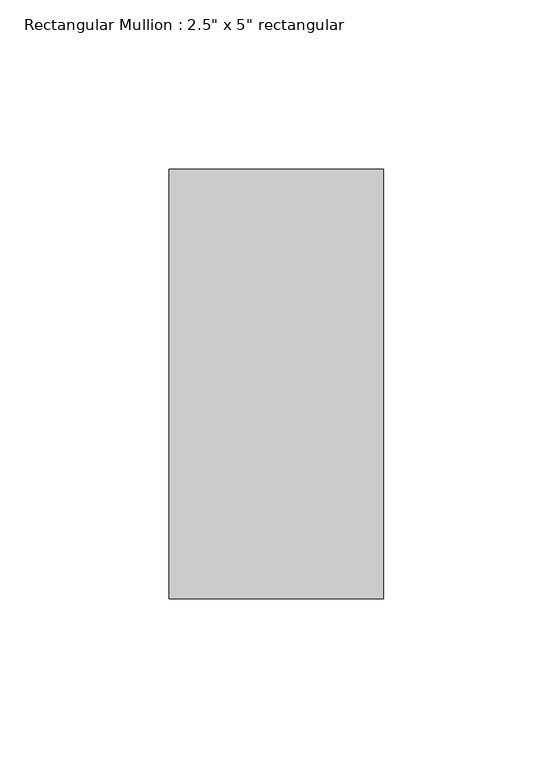
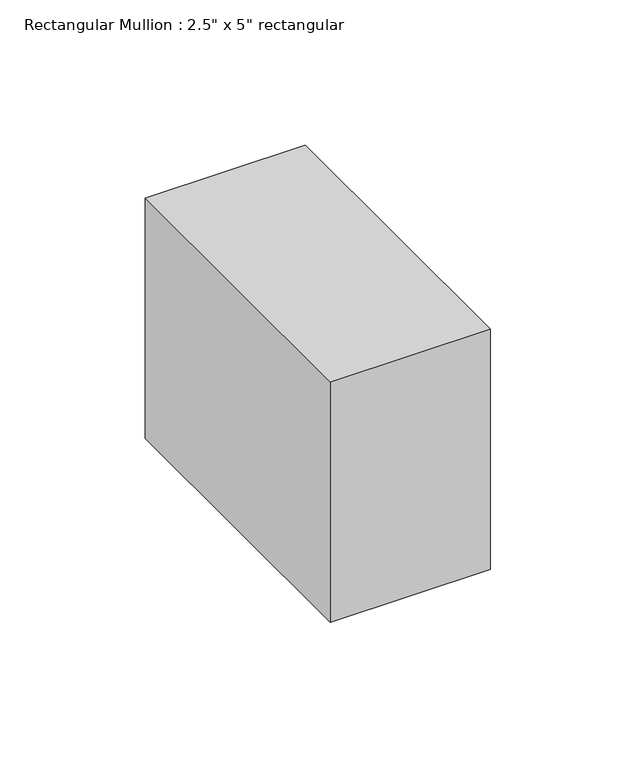
"""IFC4 building model written with IfcOpenShell, lengths in millimetres: member geometry."""

from ifc_helpers import new_model, si_unit, frame, origin, place, context, project, spatial, polyline, outline, extrude, source, transform, mapped, element, save


def member_5446ee95(model_context):
    return source(origin(), model_context, "Body", "SweptSolid", [
        extrude(outline(polyline([(0.0, 63.5), (0.0, -63.5), (-63.5, -63.5), (-63.5, 63.5), (0.0, 63.5)])), frame((0.0, 0.0, -100.9047277), z_axis=(0.0, 0.0, 1.0), x_axis=(1.0, 0.0, 0.0)), (0.0, 0.0, 1.0), 100.9047277),
    ])


if __name__ == "__main__":
    model = new_model("IFC4")
    model_context = context("Model", 3, world=origin())
    ifc_project = project(units=[si_unit("LENGTHUNIT", "METRE", prefix="MILLI")], contexts=[model_context])
    site = spatial("IfcSite", under=ifc_project)
    building = spatial("IfcBuilding", under=site)
    placement = place(None, origin())
    member_shape = member_5446ee95(model_context)
    element("IfcMember", 1, ObjectType="Rectangular Mullion : 2.5\" x 5\" rectangular", at=placement, inside=building, context=model_context, shape_type="MappedRepresentation", body=[
        mapped(member_shape, transform((0.0, 0.0, 0.0), x_axis=(1.0, 0.0, 0.0), y_axis=(0.0, 1.0, 0.0), z_axis=(0.0, 0.0, 1.0))),
    ])
    save(model, "model.ifc")

# Revit data of these elements
# Type "Rectangular Mullion : 2.5\" x 5\" rectangular"
#   built-in parameter 1007304 = 0.416667 (stored number, unit not read)
#   built-in parameter 1007301 = 0.104167 (stored number, unit not read)
#   built-in parameter 1007300 = 0.104167 (stored number, unit not read)
# Element 1 (IfcMember, "Rectangular Mullion : 2.5\" x 5\" rectangular")
#   Materials on its faces: "Aluminum"
# Materials
#   "Aluminum": class "Metal", colour RGB 247 247 247, transparency 0, Description = "Aluminum 6061", Cost = 0
